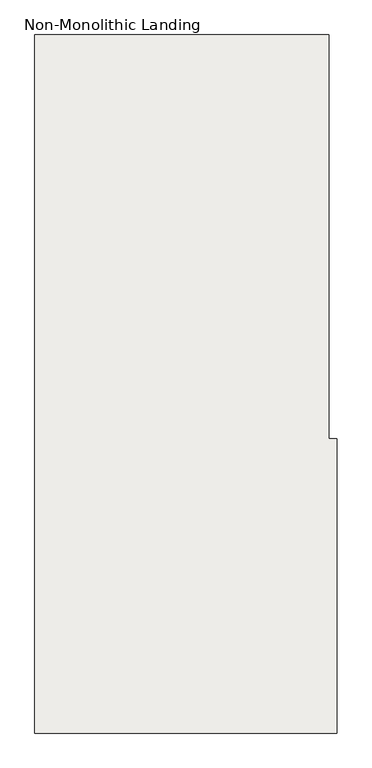
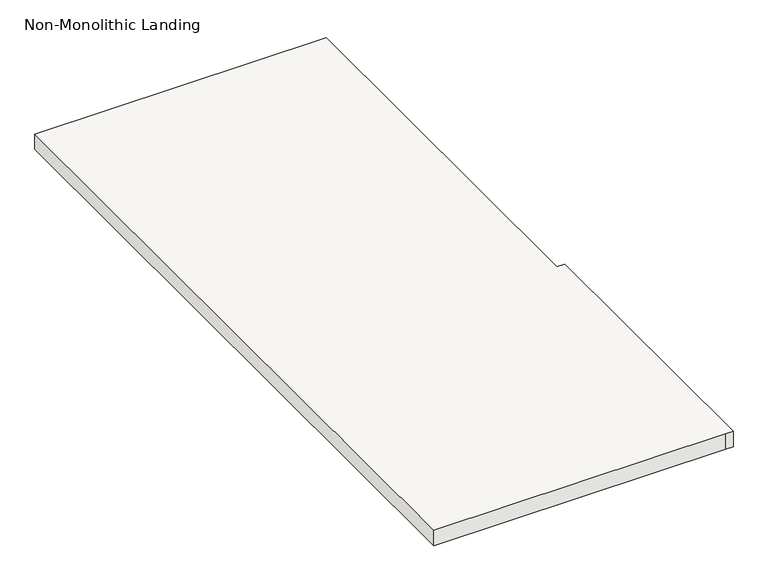
"""IFC4 building model written with IfcOpenShell, lengths in millimetres: slab geometry, Non-Monolithic Landing."""

from ifc_helpers import new_model, si_unit, origin, place, context, project, spatial, faceted_brep, source, transform, mapped, element, save


def non_monolithic_landing_543f77e1(model_context):
    return source(origin(), model_context, "Body", "Brep", [
        faceted_brep([(-12083.8120641, -2647.9669819, 11944.35), (-12058.4120641, -2647.9669819, 11969.75), (-12058.4120641, -3562.3669819, 11969.75), (-12083.8120641, -3562.3669819, 11944.35), (-12972.8120641, -2647.9669819, 11988.8), (-12972.8120641, -4817.9038196, 11988.8), (-12058.4120641, -4817.9038196, 11988.8), (-12033.0120641, -4817.9038196, 11988.8), (-12033.0120641, -3903.5038196, 11988.8), (-12058.4120641, -3903.5038196, 11988.8), (-12058.4120641, -2647.9669819, 11988.8), (-12083.8120641, -3562.3669819, 11938.0), (-12058.4120641, -3562.3669819, 11938.0), (-12058.4120641, -3903.5038196, 11938.0), (-12033.0120641, -3903.5038196, 11938.0), (-12033.0120641, -4817.9038196, 11938.0), (-12058.4120641, -4817.9038196, 11938.0), (-12972.8120641, -4817.9038196, 11938.0), (-12972.8120641, -2647.9669819, 11938.0), (-12083.8120641, -2647.9669819, 11938.0)], [[[0, 1, 2, 3]], [[4, 5, 6, 7, 8, 9, 10]], [[11, 12, 13, 14, 15, 16, 17, 18, 19]], [[12, 11, 3, 2]], [[11, 19, 0, 3]], [[4, 10, 1, 0, 19, 18]], [[5, 4, 18, 17]], [[6, 5, 17, 16]], [[7, 6, 16, 15]], [[8, 7, 15, 14]], [[9, 8, 14, 13]], [[10, 9, 13, 12, 2, 1]]]),
    ])


if __name__ == "__main__":
    model = new_model("IFC4")
    model_context = context("Model", 3, world=origin())
    ifc_project = project(units=[si_unit("LENGTHUNIT", "METRE", prefix="MILLI")], contexts=[model_context])
    site = spatial("IfcSite", under=ifc_project)
    building = spatial("IfcBuilding", under=site)
    placement = place(None, origin())
    non_monolithic_landing_shape = non_monolithic_landing_543f77e1(model_context)
    element("IfcSlab", 1, ObjectType="Non-Monolithic Landing", at=placement, inside=building, context=model_context, shape_type="MappedRepresentation", body=[
        mapped(non_monolithic_landing_shape, transform((0.0, 0.0, 0.0), x_axis=(1.0, 0.0, 0.0), y_axis=(0.0, 1.0, 0.0), z_axis=(0.0, 0.0, 1.0))),
    ])
    save(model, "model.ifc")
